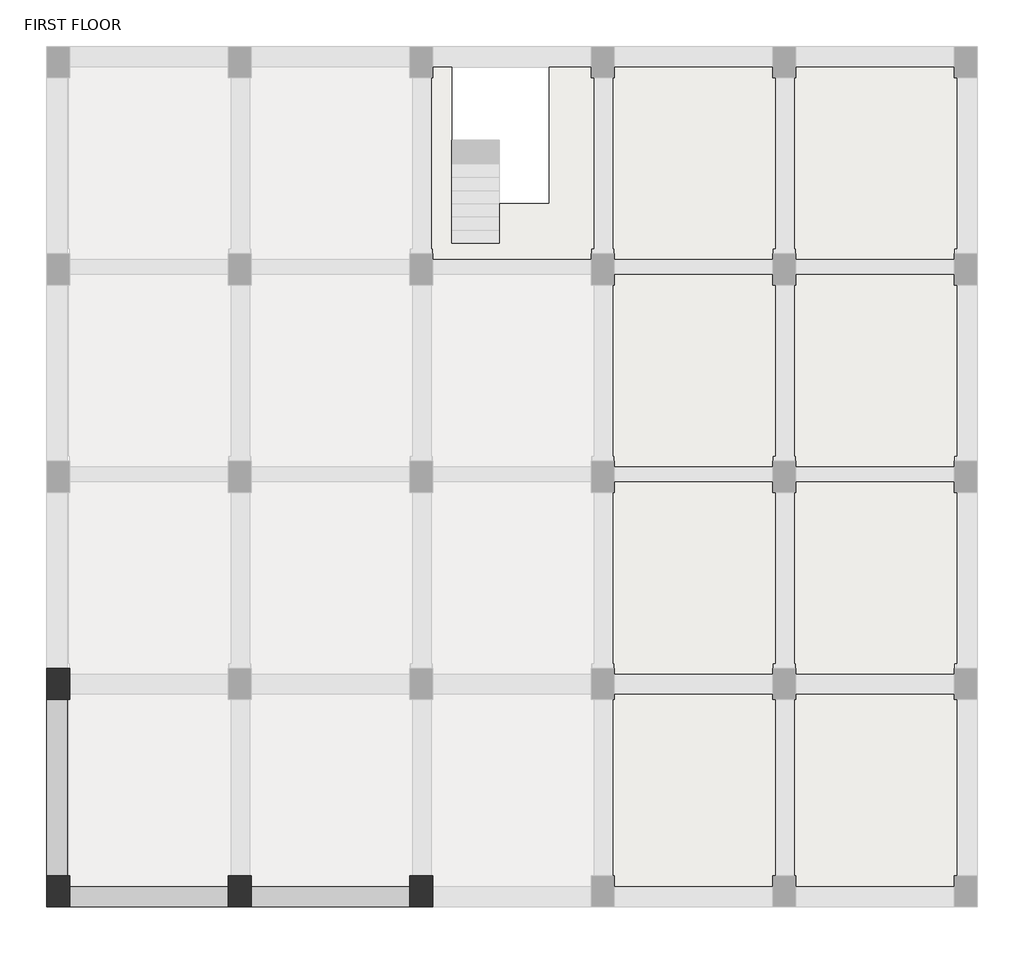
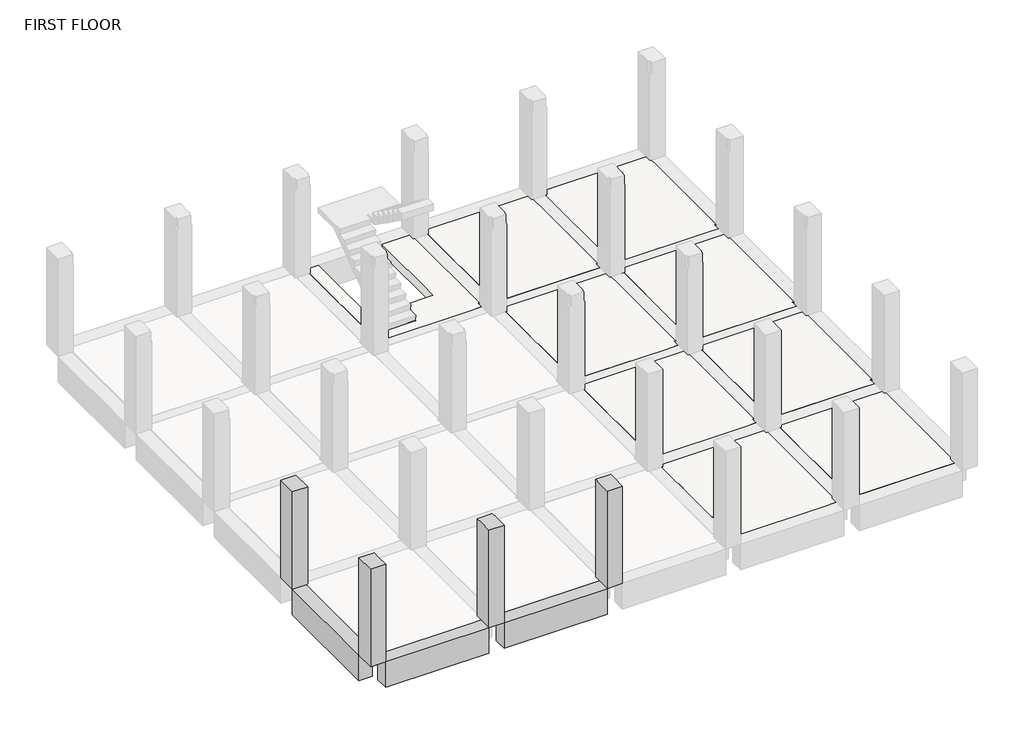
# One storey, part 2 of 4: 19 slabs, 4 columns, 3 beams.
"""IFC4 building model written with IfcOpenShell, lengths in millimetres."""

from ifc_helpers import new_model, si_unit, frame, origin, place, context, project, spatial, polyline, outline, extrude, faceted_brep, element, save

model = new_model("IFC4")

# Units and contexts
model_context = context("Model", 3, world=origin())
ifc_project = project(units=[si_unit("LENGTHUNIT", "METRE", prefix="MILLI")], contexts=[model_context])

# Site, building, storey
site = spatial("IfcSite", under=ifc_project)
building = spatial("IfcBuilding", under=site)
storey = spatial("IfcBuildingStorey", under=building, Name="FIRST FLOOR", Elevation=3048.0)

# Beams
placement = place(None, origin())
element("IfcBeam", 1, ObjectType="M_Concrete-Rectangular Beam : 400 x 800mm", at=placement, inside=storey, context=model_context, shape_type="Brep", body=[
    faceted_brep([(-5644.8884094, 3503.1212443, 3048.0), (-5644.8884094, 3103.1212443, 3048.0), (-2594.8884094, 3103.1212443, 3048.0), (-2594.8884094, 3503.1212443, 3048.0), (-5644.8884094, 3503.1212443, 2248.0), (-5644.8884094, 3503.1212443, 2748.0), (-2594.8884094, 3503.1212443, 2748.0), (-2594.8884094, 3503.1212443, 2248.0), (-5644.8884094, 3103.1212443, 2248.0), (-2594.8884094, 3103.1212443, 2248.0)], [[[0, 1, 2, 3]], [[4, 5, 0, 3, 6, 7]], [[8, 4, 7, 9]], [[1, 8, 9, 2]], [[1, 0, 5, 4, 8]], [[3, 2, 9, 7, 6]]]),
])
element("IfcBeam", 2, ObjectType="M_Concrete-Rectangular Beam : 400 x 800mm", at=placement, inside=storey, context=model_context, shape_type="Brep", body=[
    faceted_brep([(-9144.8884094, 3503.1212443, 3048.0), (-9144.8884094, 3103.1212443, 3048.0), (-6094.8884094, 3103.1212443, 3048.0), (-6094.8884094, 3503.1212443, 3048.0), (-9144.8884094, 3503.1212443, 2248.0), (-9144.8884094, 3503.1212443, 2748.0), (-6094.8884094, 3503.1212443, 2748.0), (-6094.8884094, 3503.1212443, 2248.0), (-9144.8884094, 3103.1212443, 2248.0), (-6094.8884094, 3103.1212443, 2248.0)], [[[0, 1, 2, 3]], [[4, 5, 0, 3, 6, 7]], [[8, 4, 7, 9]], [[1, 8, 9, 2]], [[1, 0, 5, 4, 8]], [[3, 2, 9, 7, 6]]]),
])
element("IfcBeam", 3, ObjectType="M_Concrete-Rectangular Beam : 400 x 800mm", at=placement, inside=storey, context=model_context, shape_type="SweptSolid", body=[
    extrude(outline(polyline([(-9594.8884094, 7103.1212443), (-9194.8884094, 7103.1212443), (-9194.8884094, 3703.1212443), (-9594.8884094, 3703.1212443), (-9594.8884094, 7103.1212443)])), frame((0.0, 0.0, 2248.0), z_axis=(0.0, 0.0, 1.0), x_axis=(1.0, 0.0, 0.0)), (0.0, 0.0, 1.0), 800.0),
])

# Columns
element("IfcColumn", 4, ObjectType="M_Concrete-Rectangular-Column : 450 x 600mm", at=placement, inside=storey, context=model_context, shape_type="Brep", body=[
    faceted_brep([(-9144.8884094, 7703.1212443, 3048.0), (-9144.8884094, 7103.1212443, 3048.0), (-9594.8884094, 7103.1212443, 3048.0), (-9594.8884094, 7703.1212443, 3048.0), (-9144.8884094, 7703.1212443, 5796.0), (-9144.8884094, 7703.1212443, 6096.0), (-9144.8884094, 7603.1212443, 6096.0), (-9144.8884094, 7203.1212443, 6096.0), (-9144.8884094, 7103.1212443, 6096.0), (-9144.8884094, 7103.1212443, 5796.0), (-9169.8884094, 7103.1212443, 6096.0), (-9594.8884094, 7103.1212443, 6096.0), (-9594.8884094, 7703.1212443, 6096.0)], [[[0, 1, 2, 3]], [[1, 0, 4, 5, 6, 7, 8, 9]], [[2, 1, 9, 8, 10, 11]], [[3, 2, 11, 12]], [[0, 3, 12, 5, 4]], [[12, 11, 10, 8, 7, 6, 5]]]),
])
element("IfcColumn", 5, ObjectType="M_Concrete-Rectangular-Column : 450 x 600mm", at=placement, inside=storey, context=model_context, shape_type="Brep", body=[
    faceted_brep([(-9144.8884094, 3703.1212443, 3048.0), (-9144.8884094, 3103.1212443, 3048.0), (-9594.8884094, 3103.1212443, 3048.0), (-9594.8884094, 3703.1212443, 3048.0), (-9144.8884094, 3703.1212443, 5796.0), (-9144.8884094, 3703.1212443, 6096.0), (-9144.8884094, 3503.1212443, 6096.0), (-9144.8884094, 3103.1212443, 6096.0), (-9594.8884094, 3103.1212443, 6096.0), (-9594.8884094, 3703.1212443, 6096.0), (-9169.8884094, 3703.1212443, 6096.0)], [[[0, 1, 2, 3]], [[1, 0, 4, 5, 6, 7]], [[2, 1, 7, 8]], [[3, 2, 8, 9]], [[0, 3, 9, 10, 5, 4]], [[8, 7, 6, 5, 10, 9]]]),
])
element("IfcColumn", 6, ObjectType="M_Concrete-Rectangular-Column : 450 x 600mm", at=placement, inside=storey, context=model_context, shape_type="Brep", body=[
    faceted_brep([(-5644.8884094, 3703.1212443, 3048.0), (-5644.8884094, 3103.1212443, 3048.0), (-6094.8884094, 3103.1212443, 3048.0), (-6094.8884094, 3703.1212443, 3048.0), (-5644.8884094, 3703.1212443, 5796.0), (-5644.8884094, 3703.1212443, 6096.0), (-5644.8884094, 3503.1212443, 6096.0), (-5644.8884094, 3103.1212443, 6096.0), (-6094.8884094, 3103.1212443, 6096.0), (-6094.8884094, 3503.1212443, 6096.0), (-6094.8884094, 3703.1212443, 6096.0), (-6094.8884094, 3703.1212443, 5796.0), (-6044.8884094, 3703.1212443, 6096.0), (-5669.8884094, 3703.1212443, 6096.0)], [[[0, 1, 2, 3]], [[1, 0, 4, 5, 6, 7]], [[2, 1, 7, 8]], [[3, 2, 8, 9, 10, 11]], [[0, 3, 11, 10, 12, 13, 5, 4]], [[8, 7, 6, 5, 13, 12, 10, 9]]]),
])
element("IfcColumn", 7, ObjectType="M_Concrete-Rectangular-Column : 450 x 600mm", at=placement, inside=storey, context=model_context, shape_type="Brep", body=[
    faceted_brep([(-2144.8884094, 3703.1212443, 3048.0), (-2144.8884094, 3103.1212443, 3048.0), (-2594.8884094, 3103.1212443, 3048.0), (-2594.8884094, 3703.1212443, 3048.0), (-2144.8884094, 3703.1212443, 5796.0), (-2144.8884094, 3703.1212443, 6096.0), (-2144.8884094, 3503.1212443, 6096.0), (-2144.8884094, 3103.1212443, 6096.0), (-2594.8884094, 3103.1212443, 6096.0), (-2594.8884094, 3503.1212443, 6096.0), (-2594.8884094, 3703.1212443, 6096.0), (-2594.8884094, 3703.1212443, 5796.0), (-2544.8884094, 3703.1212443, 6096.0), (-2169.8884094, 3703.1212443, 6096.0)], [[[0, 1, 2, 3]], [[1, 0, 4, 5, 6, 7]], [[2, 1, 7, 8]], [[3, 2, 8, 9, 10, 11]], [[0, 3, 11, 10, 12, 13, 5, 4]], [[8, 7, 6, 5, 13, 12, 10, 9]]]),
])

# Slabs
element("IfcSlab", 8, ObjectType="Generic 300mm", at=placement, inside=storey, context=model_context, shape_type="SweptSolid", body=[
    extrude(outline(polyline([(7955.1115906, 7103.1212443), (7955.1115906, 3703.1212443), (7905.1115906, 3703.1212443), (7905.1115906, 3503.1212443), (7530.1115906, 3503.1212443), (4855.1115906, 3503.1212443), (4855.1115906, 3703.1212443), (4830.1115906, 3703.1212443), (4830.1115906, 7103.1212443), (4855.1115906, 7103.1212443), (4855.1115906, 7203.1212443), (7905.1115906, 7203.1212443), (7905.1115906, 7103.1212443), (7955.1115906, 7103.1212443)])), frame((0.0, 0.0, 2748.0), z_axis=(0.0, 0.0, 1.0), x_axis=(1.0, 0.0, 0.0)), (0.0, 0.0, 1.0), 300.0),
])
element("IfcSlab", 9, ObjectType="Generic 300mm", at=placement, inside=storey, context=model_context, shape_type="Brep", body=[
    faceted_brep([(7955.1115906, 11203.1212443, 2748.0), (7955.1115906, 11103.1212443, 2748.0), (7955.1115906, 7803.1212443, 2748.0), (7905.1115906, 7803.1212443, 2748.0), (7905.1115906, 7603.1212443, 2748.0), (7530.1115906, 7603.1212443, 2748.0), (4855.1115906, 7603.1212443, 2748.0), (4855.1115906, 7803.1212443, 2748.0), (4830.1115906, 7803.1212443, 2748.0), (4830.1115906, 11103.1212443, 2748.0), (4830.1115906, 11203.1212443, 2748.0), (4855.1115906, 11203.1212443, 2748.0), (4855.1115906, 11303.1212443, 2748.0), (7905.1115906, 11303.1212443, 2748.0), (7905.1115906, 11203.1212443, 2748.0), (7955.1115906, 11203.1212443, 3048.0), (7905.1115906, 11203.1212443, 3048.0), (7905.1115906, 11303.1212443, 3048.0), (4855.1115906, 11303.1212443, 3048.0), (4855.1115906, 11203.1212443, 3048.0), (4830.1115906, 11203.1212443, 3048.0), (4830.1115906, 11103.1212443, 3048.0), (4830.1115906, 7803.1212443, 3048.0), (4855.1115906, 7803.1212443, 3048.0), (4855.1115906, 7703.1212443, 3048.0), (4855.1115906, 7603.1212443, 3048.0), (7530.1115906, 7603.1212443, 3048.0), (7905.1115906, 7603.1212443, 3048.0), (7905.1115906, 7703.1212443, 3048.0), (7905.1115906, 7803.1212443, 3048.0), (7955.1115906, 7803.1212443, 3048.0), (7955.1115906, 11103.1212443, 3048.0)], [[[0, 1, 2, 3, 4, 5, 6, 7, 8, 9, 10, 11, 12, 13, 14]], [[15, 16, 17, 18, 19, 20, 21, 22, 23, 24, 25, 26, 27, 28, 29, 30, 31]], [[2, 1, 0, 15, 31, 30]], [[3, 2, 30, 29]], [[4, 3, 29, 28, 27]], [[5, 4, 27, 26]], [[6, 5, 26, 25]], [[7, 6, 25, 24, 23]], [[8, 7, 23, 22]], [[10, 9, 8, 22, 21, 20]], [[11, 10, 20, 19]], [[12, 11, 19, 18]], [[13, 12, 18, 17]], [[14, 13, 17, 16]], [[0, 14, 16, 15]]]),
])
element("IfcSlab", 10, ObjectType="Generic 300mm", at=placement, inside=storey, context=model_context, shape_type="Brep", body=[
    faceted_brep([(4455.1115906, 11203.1212443, 2748.0), (4455.1115906, 11103.1212443, 2748.0), (4455.1115906, 7803.1212443, 2748.0), (4430.1115906, 7803.1212443, 2748.0), (4405.1115906, 7803.1212443, 2748.0), (4405.1115906, 7603.1212443, 2748.0), (4030.1115906, 7603.1212443, 2748.0), (1355.1115906, 7603.1212443, 2748.0), (1355.1115906, 7803.1212443, 2748.0), (1330.1115906, 7803.1212443, 2748.0), (1330.1115906, 11103.1212443, 2748.0), (1330.1115906, 11203.1212443, 2748.0), (1355.1115906, 11203.1212443, 2748.0), (1355.1115906, 11303.1212443, 2748.0), (4405.1115906, 11303.1212443, 2748.0), (4405.1115906, 11203.1212443, 2748.0), (4455.1115906, 11203.1212443, 3048.0), (4405.1115906, 11203.1212443, 3048.0), (4405.1115906, 11303.1212443, 3048.0), (1355.1115906, 11303.1212443, 3048.0), (1355.1115906, 11203.1212443, 3048.0), (1330.1115906, 11203.1212443, 3048.0), (1330.1115906, 11103.1212443, 3048.0), (1330.1115906, 7803.1212443, 3048.0), (1355.1115906, 7803.1212443, 3048.0), (1355.1115906, 7703.1212443, 3048.0), (1355.1115906, 7603.1212443, 3048.0), (4030.1115906, 7603.1212443, 3048.0), (4405.1115906, 7603.1212443, 3048.0), (4405.1115906, 7703.1212443, 3048.0), (4405.1115906, 7803.1212443, 3048.0), (4430.1115906, 7803.1212443, 3048.0), (4455.1115906, 7803.1212443, 3048.0), (4455.1115906, 11103.1212443, 3048.0)], [[[0, 1, 2, 3, 4, 5, 6, 7, 8, 9, 10, 11, 12, 13, 14, 15]], [[16, 17, 18, 19, 20, 21, 22, 23, 24, 25, 26, 27, 28, 29, 30, 31, 32, 33]], [[2, 1, 0, 16, 33, 32]], [[4, 3, 2, 32, 31, 30]], [[5, 4, 30, 29, 28]], [[6, 5, 28, 27]], [[7, 6, 27, 26]], [[8, 7, 26, 25, 24]], [[9, 8, 24, 23]], [[11, 10, 9, 23, 22, 21]], [[12, 11, 21, 20]], [[13, 12, 20, 19]], [[14, 13, 19, 18]], [[15, 14, 18, 17]], [[0, 15, 17, 16]]]),
])
element("IfcSlab", 11, ObjectType="Generic 300mm", at=placement, inside=storey, context=model_context, shape_type="Brep", body=[
    faceted_brep([(4455.1115906, 7103.1212443, 2748.0), (4455.1115906, 3703.1212443, 2748.0), (4430.1115906, 3703.1212443, 2748.0), (4405.1115906, 3703.1212443, 2748.0), (4405.1115906, 3503.1212443, 2748.0), (4030.1115906, 3503.1212443, 2748.0), (1355.1115906, 3503.1212443, 2748.0), (1355.1115906, 3703.1212443, 2748.0), (1330.1115906, 3703.1212443, 2748.0), (1330.1115906, 7103.1212443, 2748.0), (1355.1115906, 7103.1212443, 2748.0), (1355.1115906, 7203.1212443, 2748.0), (4405.1115906, 7203.1212443, 2748.0), (4405.1115906, 7103.1212443, 2748.0), (4430.1115906, 7103.1212443, 2748.0), (4455.1115906, 7103.1212443, 3048.0), (4405.1115906, 7103.1212443, 3048.0), (4405.1115906, 7203.1212443, 3048.0), (1355.1115906, 7203.1212443, 3048.0), (1355.1115906, 7103.1212443, 3048.0), (1330.1115906, 7103.1212443, 3048.0), (1330.1115906, 3703.1212443, 3048.0), (1355.1115906, 3703.1212443, 3048.0), (1355.1115906, 3503.1212443, 3048.0), (4030.1115906, 3503.1212443, 3048.0), (4405.1115906, 3503.1212443, 3048.0), (4405.1115906, 3703.1212443, 3048.0), (4455.1115906, 3703.1212443, 3048.0)], [[[0, 1, 2, 3, 4, 5, 6, 7, 8, 9, 10, 11, 12, 13, 14]], [[15, 16, 17, 18, 19, 20, 21, 22, 23, 24, 25, 26, 27]], [[1, 0, 15, 27]], [[3, 2, 1, 27, 26]], [[4, 3, 26, 25]], [[5, 4, 25, 24]], [[6, 5, 24, 23]], [[7, 6, 23, 22]], [[8, 7, 22, 21]], [[9, 8, 21, 20]], [[10, 9, 20, 19]], [[11, 10, 19, 18]], [[12, 11, 18, 17]], [[13, 12, 17, 16]], [[0, 14, 13, 16, 15]]]),
])
element("IfcSlab", 12, ObjectType="Generic 300mm", at=placement, inside=storey, context=model_context, shape_type="Brep", body=[
    faceted_brep([(7955.1115906, 15203.1212443, 2748.0), (7955.1115906, 15103.1212443, 2748.0), (7955.1115906, 11803.1212443, 2748.0), (7905.1115906, 11803.1212443, 2748.0), (7905.1115906, 11603.1212443, 2748.0), (7530.1115906, 11603.1212443, 2748.0), (4855.1115906, 11603.1212443, 2748.0), (4855.1115906, 11803.1212443, 2748.0), (4830.1115906, 11803.1212443, 2748.0), (4830.1115906, 15103.1212443, 2748.0), (4830.1115906, 15203.1212443, 2748.0), (4855.1115906, 15203.1212443, 2748.0), (4855.1115906, 15303.1212443, 2748.0), (7905.1115906, 15303.1212443, 2748.0), (7905.1115906, 15203.1212443, 2748.0), (7955.1115906, 15203.1212443, 3048.0), (7905.1115906, 15203.1212443, 3048.0), (7905.1115906, 15303.1212443, 3048.0), (4855.1115906, 15303.1212443, 3048.0), (4855.1115906, 15203.1212443, 3048.0), (4830.1115906, 15203.1212443, 3048.0), (4830.1115906, 15103.1212443, 3048.0), (4830.1115906, 11803.1212443, 3048.0), (4855.1115906, 11803.1212443, 3048.0), (4855.1115906, 11703.1212443, 3048.0), (4855.1115906, 11603.1212443, 3048.0), (7530.1115906, 11603.1212443, 3048.0), (7905.1115906, 11603.1212443, 3048.0), (7905.1115906, 11703.1212443, 3048.0), (7905.1115906, 11803.1212443, 3048.0), (7955.1115906, 11803.1212443, 3048.0), (7955.1115906, 15103.1212443, 3048.0)], [[[0, 1, 2, 3, 4, 5, 6, 7, 8, 9, 10, 11, 12, 13, 14]], [[15, 16, 17, 18, 19, 20, 21, 22, 23, 24, 25, 26, 27, 28, 29, 30, 31]], [[2, 1, 0, 15, 31, 30]], [[3, 2, 30, 29]], [[4, 3, 29, 28, 27]], [[5, 4, 27, 26]], [[6, 5, 26, 25]], [[7, 6, 25, 24, 23]], [[8, 7, 23, 22]], [[10, 9, 8, 22, 21, 20]], [[11, 10, 20, 19]], [[12, 11, 19, 18]], [[13, 12, 18, 17]], [[14, 13, 17, 16]], [[0, 14, 16, 15]]]),
])
element("IfcSlab", 13, ObjectType="Generic 300mm", at=placement, inside=storey, context=model_context, shape_type="Brep", body=[
    faceted_brep([(7955.1115906, 19203.1212443, 2748.0), (7955.1115906, 19103.1212443, 2748.0), (7955.1115906, 15803.1212443, 2748.0), (7905.1115906, 15803.1212443, 2748.0), (7905.1115906, 15603.1212443, 2748.0), (7530.1115906, 15603.1212443, 2748.0), (4855.1115906, 15603.1212443, 2748.0), (4855.1115906, 15803.1212443, 2748.0), (4830.1115906, 15803.1212443, 2748.0), (4830.1115906, 19103.1212443, 2748.0), (4830.1115906, 19203.1212443, 2748.0), (4855.1115906, 19203.1212443, 2748.0), (4855.1115906, 19303.1212443, 2748.0), (7905.1115906, 19303.1212443, 2748.0), (7905.1115906, 19203.1212443, 2748.0), (7955.1115906, 19203.1212443, 3048.0), (7905.1115906, 19203.1212443, 3048.0), (7905.1115906, 19303.1212443, 3048.0), (4855.1115906, 19303.1212443, 3048.0), (4855.1115906, 19203.1212443, 3048.0), (4830.1115906, 19203.1212443, 3048.0), (4830.1115906, 19103.1212443, 3048.0), (4830.1115906, 15803.1212443, 3048.0), (4855.1115906, 15803.1212443, 3048.0), (4855.1115906, 15703.1212443, 3048.0), (4855.1115906, 15603.1212443, 3048.0), (7530.1115906, 15603.1212443, 3048.0), (7905.1115906, 15603.1212443, 3048.0), (7905.1115906, 15703.1212443, 3048.0), (7905.1115906, 15803.1212443, 3048.0), (7955.1115906, 15803.1212443, 3048.0), (7955.1115906, 19103.1212443, 3048.0)], [[[0, 1, 2, 3, 4, 5, 6, 7, 8, 9, 10, 11, 12, 13, 14]], [[15, 16, 17, 18, 19, 20, 21, 22, 23, 24, 25, 26, 27, 28, 29, 30, 31]], [[2, 1, 0, 15, 31, 30]], [[3, 2, 30, 29]], [[4, 3, 29, 28, 27]], [[5, 4, 27, 26]], [[6, 5, 26, 25]], [[7, 6, 25, 24, 23]], [[8, 7, 23, 22]], [[10, 9, 8, 22, 21, 20]], [[11, 10, 20, 19]], [[12, 11, 19, 18]], [[13, 12, 18, 17]], [[14, 13, 17, 16]], [[0, 14, 16, 15]]]),
])
element("IfcSlab", 14, ObjectType="Generic 300mm", at=placement, inside=storey, context=model_context, shape_type="Brep", body=[
    faceted_brep([(4455.1115906, 19203.1212443, 2748.0), (4455.1115906, 19103.1212443, 2748.0), (4455.1115906, 15803.1212443, 2748.0), (4430.1115906, 15803.1212443, 2748.0), (4405.1115906, 15803.1212443, 2748.0), (4405.1115906, 15603.1212443, 2748.0), (4030.1115906, 15603.1212443, 2748.0), (1355.1115906, 15603.1212443, 2748.0), (1355.1115906, 15803.1212443, 2748.0), (1330.1115906, 15803.1212443, 2748.0), (1330.1115906, 19103.1212443, 2748.0), (1330.1115906, 19203.1212443, 2748.0), (1355.1115906, 19203.1212443, 2748.0), (1355.1115906, 19303.1212443, 2748.0), (4405.1115906, 19303.1212443, 2748.0), (4405.1115906, 19203.1212443, 2748.0), (4455.1115906, 19203.1212443, 3048.0), (4405.1115906, 19203.1212443, 3048.0), (4405.1115906, 19303.1212443, 3048.0), (1355.1115906, 19303.1212443, 3048.0), (1355.1115906, 19203.1212443, 3048.0), (1330.1115906, 19203.1212443, 3048.0), (1330.1115906, 19103.1212443, 3048.0), (1330.1115906, 15803.1212443, 3048.0), (1355.1115906, 15803.1212443, 3048.0), (1355.1115906, 15703.1212443, 3048.0), (1355.1115906, 15603.1212443, 3048.0), (4030.1115906, 15603.1212443, 3048.0), (4405.1115906, 15603.1212443, 3048.0), (4405.1115906, 15703.1212443, 3048.0), (4405.1115906, 15803.1212443, 3048.0), (4430.1115906, 15803.1212443, 3048.0), (4455.1115906, 15803.1212443, 3048.0), (4455.1115906, 19103.1212443, 3048.0)], [[[0, 1, 2, 3, 4, 5, 6, 7, 8, 9, 10, 11, 12, 13, 14, 15]], [[16, 17, 18, 19, 20, 21, 22, 23, 24, 25, 26, 27, 28, 29, 30, 31, 32, 33]], [[2, 1, 0, 16, 33, 32]], [[4, 3, 2, 32, 31, 30]], [[5, 4, 30, 29, 28]], [[6, 5, 28, 27]], [[7, 6, 27, 26]], [[8, 7, 26, 25, 24]], [[9, 8, 24, 23]], [[11, 10, 9, 23, 22, 21]], [[12, 11, 21, 20]], [[13, 12, 20, 19]], [[14, 13, 19, 18]], [[15, 14, 18, 17]], [[0, 15, 17, 16]]]),
])
element("IfcSlab", 15, ObjectType="Generic 300mm", at=placement, inside=storey, context=model_context, shape_type="Brep", body=[
    faceted_brep([(4455.1115906, 15203.1212443, 2748.0), (4455.1115906, 15103.1212443, 2748.0), (4455.1115906, 11803.1212443, 2748.0), (4430.1115906, 11803.1212443, 2748.0), (4405.1115906, 11803.1212443, 2748.0), (4405.1115906, 11603.1212443, 2748.0), (4030.1115906, 11603.1212443, 2748.0), (1355.1115906, 11603.1212443, 2748.0), (1355.1115906, 11803.1212443, 2748.0), (1330.1115906, 11803.1212443, 2748.0), (1330.1115906, 15103.1212443, 2748.0), (1330.1115906, 15203.1212443, 2748.0), (1355.1115906, 15203.1212443, 2748.0), (1355.1115906, 15303.1212443, 2748.0), (4405.1115906, 15303.1212443, 2748.0), (4405.1115906, 15203.1212443, 2748.0), (4455.1115906, 15203.1212443, 3048.0), (4405.1115906, 15203.1212443, 3048.0), (4405.1115906, 15303.1212443, 3048.0), (1355.1115906, 15303.1212443, 3048.0), (1355.1115906, 15203.1212443, 3048.0), (1330.1115906, 15203.1212443, 3048.0), (1330.1115906, 15103.1212443, 3048.0), (1330.1115906, 11803.1212443, 3048.0), (1355.1115906, 11803.1212443, 3048.0), (1355.1115906, 11703.1212443, 3048.0), (1355.1115906, 11603.1212443, 3048.0), (4030.1115906, 11603.1212443, 3048.0), (4405.1115906, 11603.1212443, 3048.0), (4405.1115906, 11703.1212443, 3048.0), (4405.1115906, 11803.1212443, 3048.0), (4430.1115906, 11803.1212443, 3048.0), (4455.1115906, 11803.1212443, 3048.0), (4455.1115906, 15103.1212443, 3048.0)], [[[0, 1, 2, 3, 4, 5, 6, 7, 8, 9, 10, 11, 12, 13, 14, 15]], [[16, 17, 18, 19, 20, 21, 22, 23, 24, 25, 26, 27, 28, 29, 30, 31, 32, 33]], [[2, 1, 0, 16, 33, 32]], [[4, 3, 2, 32, 31, 30]], [[5, 4, 30, 29, 28]], [[6, 5, 28, 27]], [[7, 6, 27, 26]], [[8, 7, 26, 25, 24]], [[9, 8, 24, 23]], [[11, 10, 9, 23, 22, 21]], [[12, 11, 21, 20]], [[13, 12, 20, 19]], [[14, 13, 19, 18]], [[15, 14, 18, 17]], [[0, 15, 17, 16]]]),
])
element("IfcSlab", 16, ObjectType="Generic 300mm", at=placement, inside=storey, context=model_context, shape_type="Brep", body=[
    faceted_brep([(955.1115906, 19203.1212443, 2748.0), (955.1115906, 19103.1212443, 2748.0), (955.1115906, 15803.1212443, 2748.0), (930.1115906, 15803.1212443, 2748.0), (905.1115906, 15803.1212443, 2748.0), (905.1115906, 15603.1212443, 2748.0), (530.1115906, 15603.1212443, 2748.0), (-2144.8884094, 15603.1212443, 2748.0), (-2144.8884094, 15803.1212443, 2748.0), (-2169.8884094, 15803.1212443, 2748.0), (-2169.8884094, 19103.1212443, 2748.0), (-2169.8884094, 19203.1212443, 2748.0), (-2144.8884094, 19203.1212443, 2748.0), (-2144.8884094, 19303.1212443, 2748.0), (-1784.8884094, 19303.1212443, 2748.0), (-1784.8884094, 15908.7212443, 2748.0), (-870.4884094, 15908.7212443, 2748.0), (-870.4884094, 16670.7212443, 2748.0), (-819.6884094, 16670.7212443, 2748.0), (94.7115906, 16670.7212443, 2748.0), (94.7115906, 19303.1212443, 2748.0), (905.1115906, 19303.1212443, 2748.0), (905.1115906, 19203.1212443, 2748.0), (955.1115906, 15803.1212443, 3048.0), (955.1115906, 19103.1212443, 3048.0), (955.1115906, 19203.1212443, 3048.0), (905.1115906, 19203.1212443, 3048.0), (905.1115906, 19303.1212443, 3048.0), (94.7115906, 19303.1212443, 3048.0), (94.7115906, 16670.7212443, 3048.0), (-819.6884094, 16670.7212443, 3048.0), (-870.4884094, 16670.7212443, 3048.0), (-870.4884094, 15908.7212443, 3048.0), (-1784.8884094, 15908.7212443, 3048.0), (-1784.8884094, 19303.1212443, 3048.0), (-2144.8884094, 19303.1212443, 3048.0), (-2144.8884094, 19203.1212443, 3048.0), (-2169.8884094, 19203.1212443, 3048.0), (-2169.8884094, 19103.1212443, 3048.0), (-2169.8884094, 15803.1212443, 3048.0), (-2144.8884094, 15803.1212443, 3048.0), (-2144.8884094, 15703.1212443, 3048.0), (-2144.8884094, 15603.1212443, 3048.0), (530.1115906, 15603.1212443, 3048.0), (905.1115906, 15603.1212443, 3048.0), (905.1115906, 15703.1212443, 3048.0), (905.1115906, 15803.1212443, 3048.0), (930.1115906, 15803.1212443, 3048.0)], [[[0, 1, 2, 3, 4, 5, 6, 7, 8, 9, 10, 11, 12, 13, 14, 15, 16, 17, 18, 19, 20, 21, 22]], [[23, 24, 25, 26, 27, 28, 29, 30, 31, 32, 33, 34, 35, 36, 37, 38, 39, 40, 41, 42, 43, 44, 45, 46, 47]], [[2, 1, 0, 25, 24, 23]], [[4, 3, 2, 23, 47, 46]], [[5, 4, 46, 45, 44]], [[6, 5, 44, 43]], [[7, 6, 43, 42]], [[8, 7, 42, 41, 40]], [[9, 8, 40, 39]], [[11, 10, 9, 39, 38, 37]], [[12, 11, 37, 36]], [[13, 12, 36, 35]], [[13, 35, 34, 14]], [[27, 21, 20, 28]], [[22, 21, 27, 26]], [[0, 22, 26, 25]], [[19, 29, 28, 20]], [[33, 15, 14, 34]], [[15, 33, 32, 16]], [[16, 32, 31, 17]], [[17, 31, 30, 18]], [[29, 19, 18, 30]]]),
])
element("IfcSlab", 17, ObjectType="Generic 300mm", at=placement, inside=storey, context=model_context, shape_type="SweptSolid", body=[
    extrude(outline(polyline([(7955.1115906, 7103.1212443), (7955.1115906, 3703.1212443), (7905.1115906, 3703.1212443), (7905.1115906, 3503.1212443), (7530.1115906, 3503.1212443), (4855.1115906, 3503.1212443), (4855.1115906, 3703.1212443), (4830.1115906, 3703.1212443), (4830.1115906, 7103.1212443), (4855.1115906, 7103.1212443), (4855.1115906, 7203.1212443), (7905.1115906, 7203.1212443), (7905.1115906, 7103.1212443), (7955.1115906, 7103.1212443)])), frame((0.0, 0.0, 2748.0), z_axis=(0.0, 0.0, 1.0), x_axis=(1.0, 0.0, 0.0)), (0.0, 0.0, 1.0), 300.0),
])
element("IfcSlab", 18, ObjectType="Generic 300mm", at=placement, inside=storey, context=model_context, shape_type="Brep", body=[
    faceted_brep([(7955.1115906, 11203.1212443, 2748.0), (7955.1115906, 11103.1212443, 2748.0), (7955.1115906, 7803.1212443, 2748.0), (7905.1115906, 7803.1212443, 2748.0), (7905.1115906, 7603.1212443, 2748.0), (7530.1115906, 7603.1212443, 2748.0), (4855.1115906, 7603.1212443, 2748.0), (4855.1115906, 7803.1212443, 2748.0), (4830.1115906, 7803.1212443, 2748.0), (4830.1115906, 11103.1212443, 2748.0), (4830.1115906, 11203.1212443, 2748.0), (4855.1115906, 11203.1212443, 2748.0), (4855.1115906, 11303.1212443, 2748.0), (7905.1115906, 11303.1212443, 2748.0), (7905.1115906, 11203.1212443, 2748.0), (7955.1115906, 11203.1212443, 3048.0), (7905.1115906, 11203.1212443, 3048.0), (7905.1115906, 11303.1212443, 3048.0), (4855.1115906, 11303.1212443, 3048.0), (4855.1115906, 11203.1212443, 3048.0), (4830.1115906, 11203.1212443, 3048.0), (4830.1115906, 11103.1212443, 3048.0), (4830.1115906, 7803.1212443, 3048.0), (4855.1115906, 7803.1212443, 3048.0), (4855.1115906, 7703.1212443, 3048.0), (4855.1115906, 7603.1212443, 3048.0), (7530.1115906, 7603.1212443, 3048.0), (7905.1115906, 7603.1212443, 3048.0), (7905.1115906, 7703.1212443, 3048.0), (7905.1115906, 7803.1212443, 3048.0), (7955.1115906, 7803.1212443, 3048.0), (7955.1115906, 11103.1212443, 3048.0)], [[[0, 1, 2, 3, 4, 5, 6, 7, 8, 9, 10, 11, 12, 13, 14]], [[15, 16, 17, 18, 19, 20, 21, 22, 23, 24, 25, 26, 27, 28, 29, 30, 31]], [[2, 1, 0, 15, 31, 30]], [[3, 2, 30, 29]], [[4, 3, 29, 28, 27]], [[5, 4, 27, 26]], [[6, 5, 26, 25]], [[7, 6, 25, 24, 23]], [[8, 7, 23, 22]], [[10, 9, 8, 22, 21, 20]], [[11, 10, 20, 19]], [[12, 11, 19, 18]], [[13, 12, 18, 17]], [[14, 13, 17, 16]], [[0, 14, 16, 15]]]),
])
element("IfcSlab", 19, ObjectType="Generic 300mm", at=placement, inside=storey, context=model_context, shape_type="Brep", body=[
    faceted_brep([(4455.1115906, 11203.1212443, 2748.0), (4455.1115906, 11103.1212443, 2748.0), (4455.1115906, 7803.1212443, 2748.0), (4430.1115906, 7803.1212443, 2748.0), (4405.1115906, 7803.1212443, 2748.0), (4405.1115906, 7603.1212443, 2748.0), (4030.1115906, 7603.1212443, 2748.0), (1355.1115906, 7603.1212443, 2748.0), (1355.1115906, 7803.1212443, 2748.0), (1330.1115906, 7803.1212443, 2748.0), (1330.1115906, 11103.1212443, 2748.0), (1330.1115906, 11203.1212443, 2748.0), (1355.1115906, 11203.1212443, 2748.0), (1355.1115906, 11303.1212443, 2748.0), (4405.1115906, 11303.1212443, 2748.0), (4405.1115906, 11203.1212443, 2748.0), (4455.1115906, 11203.1212443, 3048.0), (4405.1115906, 11203.1212443, 3048.0), (4405.1115906, 11303.1212443, 3048.0), (1355.1115906, 11303.1212443, 3048.0), (1355.1115906, 11203.1212443, 3048.0), (1330.1115906, 11203.1212443, 3048.0), (1330.1115906, 11103.1212443, 3048.0), (1330.1115906, 7803.1212443, 3048.0), (1355.1115906, 7803.1212443, 3048.0), (1355.1115906, 7703.1212443, 3048.0), (1355.1115906, 7603.1212443, 3048.0), (4030.1115906, 7603.1212443, 3048.0), (4405.1115906, 7603.1212443, 3048.0), (4405.1115906, 7703.1212443, 3048.0), (4405.1115906, 7803.1212443, 3048.0), (4430.1115906, 7803.1212443, 3048.0), (4455.1115906, 7803.1212443, 3048.0), (4455.1115906, 11103.1212443, 3048.0)], [[[0, 1, 2, 3, 4, 5, 6, 7, 8, 9, 10, 11, 12, 13, 14, 15]], [[16, 17, 18, 19, 20, 21, 22, 23, 24, 25, 26, 27, 28, 29, 30, 31, 32, 33]], [[2, 1, 0, 16, 33, 32]], [[4, 3, 2, 32, 31, 30]], [[5, 4, 30, 29, 28]], [[6, 5, 28, 27]], [[7, 6, 27, 26]], [[8, 7, 26, 25, 24]], [[9, 8, 24, 23]], [[11, 10, 9, 23, 22, 21]], [[12, 11, 21, 20]], [[13, 12, 20, 19]], [[14, 13, 19, 18]], [[15, 14, 18, 17]], [[0, 15, 17, 16]]]),
])
element("IfcSlab", 20, ObjectType="Generic 300mm", at=placement, inside=storey, context=model_context, shape_type="Brep", body=[
    faceted_brep([(4455.1115906, 7103.1212443, 2748.0), (4455.1115906, 3703.1212443, 2748.0), (4430.1115906, 3703.1212443, 2748.0), (4405.1115906, 3703.1212443, 2748.0), (4405.1115906, 3503.1212443, 2748.0), (4030.1115906, 3503.1212443, 2748.0), (1355.1115906, 3503.1212443, 2748.0), (1355.1115906, 3703.1212443, 2748.0), (1330.1115906, 3703.1212443, 2748.0), (1330.1115906, 7103.1212443, 2748.0), (1355.1115906, 7103.1212443, 2748.0), (1355.1115906, 7203.1212443, 2748.0), (4405.1115906, 7203.1212443, 2748.0), (4405.1115906, 7103.1212443, 2748.0), (4430.1115906, 7103.1212443, 2748.0), (4455.1115906, 7103.1212443, 3048.0), (4405.1115906, 7103.1212443, 3048.0), (4405.1115906, 7203.1212443, 3048.0), (1355.1115906, 7203.1212443, 3048.0), (1355.1115906, 7103.1212443, 3048.0), (1330.1115906, 7103.1212443, 3048.0), (1330.1115906, 3703.1212443, 3048.0), (1355.1115906, 3703.1212443, 3048.0), (1355.1115906, 3503.1212443, 3048.0), (4030.1115906, 3503.1212443, 3048.0), (4405.1115906, 3503.1212443, 3048.0), (4405.1115906, 3703.1212443, 3048.0), (4455.1115906, 3703.1212443, 3048.0)], [[[0, 1, 2, 3, 4, 5, 6, 7, 8, 9, 10, 11, 12, 13, 14]], [[15, 16, 17, 18, 19, 20, 21, 22, 23, 24, 25, 26, 27]], [[1, 0, 15, 27]], [[3, 2, 1, 27, 26]], [[4, 3, 26, 25]], [[5, 4, 25, 24]], [[6, 5, 24, 23]], [[7, 6, 23, 22]], [[8, 7, 22, 21]], [[9, 8, 21, 20]], [[10, 9, 20, 19]], [[11, 10, 19, 18]], [[12, 11, 18, 17]], [[13, 12, 17, 16]], [[0, 14, 13, 16, 15]]]),
])
element("IfcSlab", 21, ObjectType="Generic 300mm", at=placement, inside=storey, context=model_context, shape_type="Brep", body=[
    faceted_brep([(7955.1115906, 15203.1212443, 2748.0), (7955.1115906, 15103.1212443, 2748.0), (7955.1115906, 11803.1212443, 2748.0), (7905.1115906, 11803.1212443, 2748.0), (7905.1115906, 11603.1212443, 2748.0), (7530.1115906, 11603.1212443, 2748.0), (4855.1115906, 11603.1212443, 2748.0), (4855.1115906, 11803.1212443, 2748.0), (4830.1115906, 11803.1212443, 2748.0), (4830.1115906, 15103.1212443, 2748.0), (4830.1115906, 15203.1212443, 2748.0), (4855.1115906, 15203.1212443, 2748.0), (4855.1115906, 15303.1212443, 2748.0), (7905.1115906, 15303.1212443, 2748.0), (7905.1115906, 15203.1212443, 2748.0), (7955.1115906, 15203.1212443, 3048.0), (7905.1115906, 15203.1212443, 3048.0), (7905.1115906, 15303.1212443, 3048.0), (4855.1115906, 15303.1212443, 3048.0), (4855.1115906, 15203.1212443, 3048.0), (4830.1115906, 15203.1212443, 3048.0), (4830.1115906, 15103.1212443, 3048.0), (4830.1115906, 11803.1212443, 3048.0), (4855.1115906, 11803.1212443, 3048.0), (4855.1115906, 11703.1212443, 3048.0), (4855.1115906, 11603.1212443, 3048.0), (7530.1115906, 11603.1212443, 3048.0), (7905.1115906, 11603.1212443, 3048.0), (7905.1115906, 11703.1212443, 3048.0), (7905.1115906, 11803.1212443, 3048.0), (7955.1115906, 11803.1212443, 3048.0), (7955.1115906, 15103.1212443, 3048.0)], [[[0, 1, 2, 3, 4, 5, 6, 7, 8, 9, 10, 11, 12, 13, 14]], [[15, 16, 17, 18, 19, 20, 21, 22, 23, 24, 25, 26, 27, 28, 29, 30, 31]], [[2, 1, 0, 15, 31, 30]], [[3, 2, 30, 29]], [[4, 3, 29, 28, 27]], [[5, 4, 27, 26]], [[6, 5, 26, 25]], [[7, 6, 25, 24, 23]], [[8, 7, 23, 22]], [[10, 9, 8, 22, 21, 20]], [[11, 10, 20, 19]], [[12, 11, 19, 18]], [[13, 12, 18, 17]], [[14, 13, 17, 16]], [[0, 14, 16, 15]]]),
])
element("IfcSlab", 22, ObjectType="Generic 300mm", at=placement, inside=storey, context=model_context, shape_type="Brep", body=[
    faceted_brep([(7955.1115906, 19203.1212443, 2748.0), (7955.1115906, 19103.1212443, 2748.0), (7955.1115906, 15803.1212443, 2748.0), (7905.1115906, 15803.1212443, 2748.0), (7905.1115906, 15603.1212443, 2748.0), (7530.1115906, 15603.1212443, 2748.0), (4855.1115906, 15603.1212443, 2748.0), (4855.1115906, 15803.1212443, 2748.0), (4830.1115906, 15803.1212443, 2748.0), (4830.1115906, 19103.1212443, 2748.0), (4830.1115906, 19203.1212443, 2748.0), (4855.1115906, 19203.1212443, 2748.0), (4855.1115906, 19303.1212443, 2748.0), (7905.1115906, 19303.1212443, 2748.0), (7905.1115906, 19203.1212443, 2748.0), (7955.1115906, 19203.1212443, 3048.0), (7905.1115906, 19203.1212443, 3048.0), (7905.1115906, 19303.1212443, 3048.0), (4855.1115906, 19303.1212443, 3048.0), (4855.1115906, 19203.1212443, 3048.0), (4830.1115906, 19203.1212443, 3048.0), (4830.1115906, 19103.1212443, 3048.0), (4830.1115906, 15803.1212443, 3048.0), (4855.1115906, 15803.1212443, 3048.0), (4855.1115906, 15703.1212443, 3048.0), (4855.1115906, 15603.1212443, 3048.0), (7530.1115906, 15603.1212443, 3048.0), (7905.1115906, 15603.1212443, 3048.0), (7905.1115906, 15703.1212443, 3048.0), (7905.1115906, 15803.1212443, 3048.0), (7955.1115906, 15803.1212443, 3048.0), (7955.1115906, 19103.1212443, 3048.0)], [[[0, 1, 2, 3, 4, 5, 6, 7, 8, 9, 10, 11, 12, 13, 14]], [[15, 16, 17, 18, 19, 20, 21, 22, 23, 24, 25, 26, 27, 28, 29, 30, 31]], [[2, 1, 0, 15, 31, 30]], [[3, 2, 30, 29]], [[4, 3, 29, 28, 27]], [[5, 4, 27, 26]], [[6, 5, 26, 25]], [[7, 6, 25, 24, 23]], [[8, 7, 23, 22]], [[10, 9, 8, 22, 21, 20]], [[11, 10, 20, 19]], [[12, 11, 19, 18]], [[13, 12, 18, 17]], [[14, 13, 17, 16]], [[0, 14, 16, 15]]]),
])
element("IfcSlab", 23, ObjectType="Generic 300mm", at=placement, inside=storey, context=model_context, shape_type="Brep", body=[
    faceted_brep([(4455.1115906, 19203.1212443, 2748.0), (4455.1115906, 19103.1212443, 2748.0), (4455.1115906, 15803.1212443, 2748.0), (4430.1115906, 15803.1212443, 2748.0), (4405.1115906, 15803.1212443, 2748.0), (4405.1115906, 15603.1212443, 2748.0), (4030.1115906, 15603.1212443, 2748.0), (1355.1115906, 15603.1212443, 2748.0), (1355.1115906, 15803.1212443, 2748.0), (1330.1115906, 15803.1212443, 2748.0), (1330.1115906, 19103.1212443, 2748.0), (1330.1115906, 19203.1212443, 2748.0), (1355.1115906, 19203.1212443, 2748.0), (1355.1115906, 19303.1212443, 2748.0), (4405.1115906, 19303.1212443, 2748.0), (4405.1115906, 19203.1212443, 2748.0), (4455.1115906, 19203.1212443, 3048.0), (4405.1115906, 19203.1212443, 3048.0), (4405.1115906, 19303.1212443, 3048.0), (1355.1115906, 19303.1212443, 3048.0), (1355.1115906, 19203.1212443, 3048.0), (1330.1115906, 19203.1212443, 3048.0), (1330.1115906, 19103.1212443, 3048.0), (1330.1115906, 15803.1212443, 3048.0), (1355.1115906, 15803.1212443, 3048.0), (1355.1115906, 15703.1212443, 3048.0), (1355.1115906, 15603.1212443, 3048.0), (4030.1115906, 15603.1212443, 3048.0), (4405.1115906, 15603.1212443, 3048.0), (4405.1115906, 15703.1212443, 3048.0), (4405.1115906, 15803.1212443, 3048.0), (4430.1115906, 15803.1212443, 3048.0), (4455.1115906, 15803.1212443, 3048.0), (4455.1115906, 19103.1212443, 3048.0)], [[[0, 1, 2, 3, 4, 5, 6, 7, 8, 9, 10, 11, 12, 13, 14, 15]], [[16, 17, 18, 19, 20, 21, 22, 23, 24, 25, 26, 27, 28, 29, 30, 31, 32, 33]], [[2, 1, 0, 16, 33, 32]], [[4, 3, 2, 32, 31, 30]], [[5, 4, 30, 29, 28]], [[6, 5, 28, 27]], [[7, 6, 27, 26]], [[8, 7, 26, 25, 24]], [[9, 8, 24, 23]], [[11, 10, 9, 23, 22, 21]], [[12, 11, 21, 20]], [[13, 12, 20, 19]], [[14, 13, 19, 18]], [[15, 14, 18, 17]], [[0, 15, 17, 16]]]),
])
element("IfcSlab", 24, ObjectType="Generic 300mm", at=placement, inside=storey, context=model_context, shape_type="Brep", body=[
    faceted_brep([(4455.1115906, 15203.1212443, 2748.0), (4455.1115906, 15103.1212443, 2748.0), (4455.1115906, 11803.1212443, 2748.0), (4430.1115906, 11803.1212443, 2748.0), (4405.1115906, 11803.1212443, 2748.0), (4405.1115906, 11603.1212443, 2748.0), (4030.1115906, 11603.1212443, 2748.0), (1355.1115906, 11603.1212443, 2748.0), (1355.1115906, 11803.1212443, 2748.0), (1330.1115906, 11803.1212443, 2748.0), (1330.1115906, 15103.1212443, 2748.0), (1330.1115906, 15203.1212443, 2748.0), (1355.1115906, 15203.1212443, 2748.0), (1355.1115906, 15303.1212443, 2748.0), (4405.1115906, 15303.1212443, 2748.0), (4405.1115906, 15203.1212443, 2748.0), (4455.1115906, 15203.1212443, 3048.0), (4405.1115906, 15203.1212443, 3048.0), (4405.1115906, 15303.1212443, 3048.0), (1355.1115906, 15303.1212443, 3048.0), (1355.1115906, 15203.1212443, 3048.0), (1330.1115906, 15203.1212443, 3048.0), (1330.1115906, 15103.1212443, 3048.0), (1330.1115906, 11803.1212443, 3048.0), (1355.1115906, 11803.1212443, 3048.0), (1355.1115906, 11703.1212443, 3048.0), (1355.1115906, 11603.1212443, 3048.0), (4030.1115906, 11603.1212443, 3048.0), (4405.1115906, 11603.1212443, 3048.0), (4405.1115906, 11703.1212443, 3048.0), (4405.1115906, 11803.1212443, 3048.0), (4430.1115906, 11803.1212443, 3048.0), (4455.1115906, 11803.1212443, 3048.0), (4455.1115906, 15103.1212443, 3048.0)], [[[0, 1, 2, 3, 4, 5, 6, 7, 8, 9, 10, 11, 12, 13, 14, 15]], [[16, 17, 18, 19, 20, 21, 22, 23, 24, 25, 26, 27, 28, 29, 30, 31, 32, 33]], [[2, 1, 0, 16, 33, 32]], [[4, 3, 2, 32, 31, 30]], [[5, 4, 30, 29, 28]], [[6, 5, 28, 27]], [[7, 6, 27, 26]], [[8, 7, 26, 25, 24]], [[9, 8, 24, 23]], [[11, 10, 9, 23, 22, 21]], [[12, 11, 21, 20]], [[13, 12, 20, 19]], [[14, 13, 19, 18]], [[15, 14, 18, 17]], [[0, 15, 17, 16]]]),
])
element("IfcSlab", 25, ObjectType="Generic 300mm", at=placement, inside=storey, context=model_context, shape_type="Brep", body=[
    faceted_brep([(955.1115906, 19203.1212443, 2748.0), (955.1115906, 19103.1212443, 2748.0), (955.1115906, 15803.1212443, 2748.0), (930.1115906, 15803.1212443, 2748.0), (905.1115906, 15803.1212443, 2748.0), (905.1115906, 15603.1212443, 2748.0), (530.1115906, 15603.1212443, 2748.0), (-2144.8884094, 15603.1212443, 2748.0), (-2144.8884094, 15803.1212443, 2748.0), (-2169.8884094, 15803.1212443, 2748.0), (-2169.8884094, 19103.1212443, 2748.0), (-2169.8884094, 19203.1212443, 2748.0), (-2144.8884094, 19203.1212443, 2748.0), (-2144.8884094, 19303.1212443, 2748.0), (-1784.8884094, 19303.1212443, 2748.0), (-1784.8884094, 15908.7212443, 2748.0), (-870.4884094, 15908.7212443, 2748.0), (-870.4884094, 16670.7212443, 2748.0), (-819.6884094, 16670.7212443, 2748.0), (94.7115906, 16670.7212443, 2748.0), (94.7115906, 19303.1212443, 2748.0), (905.1115906, 19303.1212443, 2748.0), (905.1115906, 19203.1212443, 2748.0), (955.1115906, 15803.1212443, 3048.0), (955.1115906, 19103.1212443, 3048.0), (955.1115906, 19203.1212443, 3048.0), (905.1115906, 19203.1212443, 3048.0), (905.1115906, 19303.1212443, 3048.0), (94.7115906, 19303.1212443, 3048.0), (94.7115906, 16670.7212443, 3048.0), (-819.6884094, 16670.7212443, 3048.0), (-870.4884094, 16670.7212443, 3048.0), (-870.4884094, 15908.7212443, 3048.0), (-1784.8884094, 15908.7212443, 3048.0), (-1784.8884094, 19303.1212443, 3048.0), (-2144.8884094, 19303.1212443, 3048.0), (-2144.8884094, 19203.1212443, 3048.0), (-2169.8884094, 19203.1212443, 3048.0), (-2169.8884094, 19103.1212443, 3048.0), (-2169.8884094, 15803.1212443, 3048.0), (-2144.8884094, 15803.1212443, 3048.0), (-2144.8884094, 15703.1212443, 3048.0), (-2144.8884094, 15603.1212443, 3048.0), (530.1115906, 15603.1212443, 3048.0), (905.1115906, 15603.1212443, 3048.0), (905.1115906, 15703.1212443, 3048.0), (905.1115906, 15803.1212443, 3048.0), (930.1115906, 15803.1212443, 3048.0)], [[[0, 1, 2, 3, 4, 5, 6, 7, 8, 9, 10, 11, 12, 13, 14, 15, 16, 17, 18, 19, 20, 21, 22]], [[23, 24, 25, 26, 27, 28, 29, 30, 31, 32, 33, 34, 35, 36, 37, 38, 39, 40, 41, 42, 43, 44, 45, 46, 47]], [[2, 1, 0, 25, 24, 23]], [[4, 3, 2, 23, 47, 46]], [[5, 4, 46, 45, 44]], [[6, 5, 44, 43]], [[7, 6, 43, 42]], [[8, 7, 42, 41, 40]], [[9, 8, 40, 39]], [[11, 10, 9, 39, 38, 37]], [[12, 11, 37, 36]], [[13, 12, 36, 35]], [[13, 35, 34, 14]], [[27, 21, 20, 28]], [[22, 21, 27, 26]], [[0, 22, 26, 25]], [[19, 29, 28, 20]], [[33, 15, 14, 34]], [[15, 33, 32, 16]], [[16, 32, 31, 17]], [[17, 31, 30, 18]], [[29, 19, 18, 30]]]),
])
element("IfcSlab", 26, ObjectType="Generic 300mm", at=placement, inside=storey, context=model_context, shape_type="Brep", body=[
    faceted_brep([(-2544.8884094, 19203.1212443, 2748.0), (-2544.8884094, 19103.1212443, 2748.0), (-2544.8884094, 15803.1212443, 2748.0), (-2569.8884094, 15803.1212443, 2748.0), (-2594.8884094, 15803.1212443, 2748.0), (-2594.8884094, 15603.1212443, 2748.0), (-2969.8884094, 15603.1212443, 2748.0), (-5644.8884094, 15603.1212443, 2748.0), (-5644.8884094, 15803.1212443, 2748.0), (-5669.8884094, 15803.1212443, 2748.0), (-5669.8884094, 19103.1212443, 2748.0), (-5669.8884094, 19203.1212443, 2748.0), (-5644.8884094, 19203.1212443, 2748.0), (-5644.8884094, 19303.1212443, 2748.0), (-2594.8884094, 19303.1212443, 2748.0), (-2594.8884094, 19203.1212443, 2748.0), (-2544.8884094, 19203.1212443, 3048.0), (-2594.8884094, 19203.1212443, 3048.0), (-2594.8884094, 19303.1212443, 3048.0), (-5644.8884094, 19303.1212443, 3048.0), (-5644.8884094, 19203.1212443, 3048.0), (-5669.8884094, 19203.1212443, 3048.0), (-5669.8884094, 19103.1212443, 3048.0), (-5669.8884094, 15803.1212443, 3048.0), (-5644.8884094, 15803.1212443, 3048.0), (-5644.8884094, 15703.1212443, 3048.0), (-5644.8884094, 15603.1212443, 3048.0), (-2969.8884094, 15603.1212443, 3048.0), (-2594.8884094, 15603.1212443, 3048.0), (-2594.8884094, 15703.1212443, 3048.0), (-2594.8884094, 15803.1212443, 3048.0), (-2569.8884094, 15803.1212443, 3048.0), (-2544.8884094, 15803.1212443, 3048.0), (-2544.8884094, 19103.1212443, 3048.0)], [[[0, 1, 2, 3, 4, 5, 6, 7, 8, 9, 10, 11, 12, 13, 14, 15]], [[16, 17, 18, 19, 20, 21, 22, 23, 24, 25, 26, 27, 28, 29, 30, 31, 32, 33]], [[2, 1, 0, 16, 33, 32]], [[4, 3, 2, 32, 31, 30]], [[5, 4, 30, 29, 28]], [[6, 5, 28, 27]], [[7, 6, 27, 26]], [[8, 7, 26, 25, 24]], [[9, 8, 24, 23]], [[11, 10, 9, 23, 22, 21]], [[12, 11, 21, 20]], [[13, 12, 20, 19]], [[14, 13, 19, 18]], [[15, 14, 18, 17]], [[0, 15, 17, 16]]]),
])

save(model, "model.ifc")

# Revit data of these elements
# Type "M_Concrete-Rectangular Beam : 400 x 800mm"
#   Length [instance default] = 5' - 0"
#   b = 1' - 3.74803"
#   h = 2' - 7.49606"
#   Structural Material [instance default] = Concrete, Cast-in-Place gray
#   Assembly Code = ""
# Type "M_Concrete-Rectangular-Column : 450 x 600mm"
#   b = 1' - 5.71654"
#   h = 1' - 11.62205"
#   Structural Material [instance default] = Concrete, Cast-in-Place gray
# Type "Generic 300mm"
#   Function = 0
#   Layers, outside or top first: 0' - 11.81102" no material (function 1)
# Elements 1, 2, 3 (IfcBeam, "M_Concrete-Rectangular Beam : 400 x 800mm")
#   Structural Material = Concrete, Cast-in-Place gray
#   Phase Created = New Construction
#   Materials on its faces: "Concrete, Cast-in-Place gray"
# Elements 4, 5, 6, 7 (IfcColumn, "M_Concrete-Rectangular-Column : 450 x 600mm")
#   Structural Material = Concrete, Cast-in-Place gray
#   Phase Created = New Construction
#   Materials on its faces: "Concrete, Cast-in-Place gray"
# Elements 8, 9, 10, 11, 12, 13, 14, 15, 16, 17, 18, 19, 20, 21, 22, 23, 24, 25, 26 (IfcSlab, "Generic 300mm")
#   built-in parameter 1001955 = 1.5708 (stored number, unit not read)
#   Height Offset From Level = 0' - 0"
#   built-in parameter 1001954 = 1
#   Phase Created = New Construction
#   Materials on its faces: "Default Floor"
# Materials
#   "Concrete, Cast-in-Place gray": class "Concrete", colour RGB 192 192 192, transparency 0, Description = "Cast-in-place concrete", Cost = 0
#   "Default Floor": colour RGB 127 127 127, transparency 0, Cost = 0
